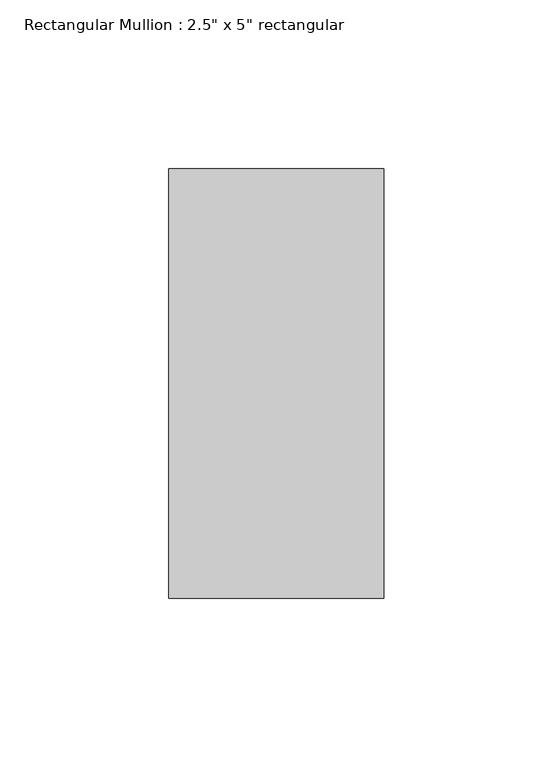
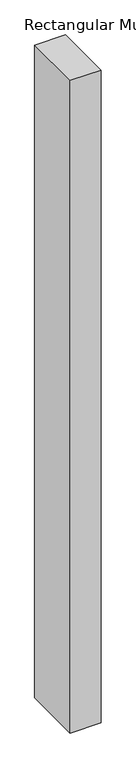
"""IFC4 building model written with IfcOpenShell, lengths in millimetres: member geometry."""

from ifc_helpers import new_model, si_unit, frame, origin, place, context, project, spatial, polyline, outline, extrude, source, transform, mapped, element, save


def member_3c30aa5e(model_context):
    return source(origin(), model_context, "Body", "SweptSolid", [
        extrude(outline(polyline([(31.75, 63.5), (31.75, -63.5), (-31.75, -63.5), (-31.75, 63.5), (31.75, 63.5)])), frame((0.0, 0.0, -1426.6333333), z_axis=(0.0, 0.0, 1.0), x_axis=(1.0, 0.0, 0.0)), (0.0, 0.0, 1.0), 1426.6333333),
    ])


if __name__ == "__main__":
    model = new_model("IFC4")
    model_context = context("Model", 3, world=origin())
    ifc_project = project(units=[si_unit("LENGTHUNIT", "METRE", prefix="MILLI")], contexts=[model_context])
    site = spatial("IfcSite", under=ifc_project)
    building = spatial("IfcBuilding", under=site)
    placement = place(None, origin())
    member_shape = member_3c30aa5e(model_context)
    element("IfcMember", 1, ObjectType="Rectangular Mullion : 2.5\" x 5\" rectangular", at=placement, inside=building, context=model_context, shape_type="MappedRepresentation", body=[
        mapped(member_shape, transform((0.0, 0.0, 0.0), x_axis=(1.0, 0.0, 0.0), y_axis=(0.0, 1.0, 0.0), z_axis=(0.0, 0.0, 1.0))),
    ])
    save(model, "model.ifc")

# Revit data of these elements
# Type "Rectangular Mullion : 2.5\" x 5\" rectangular"
#   built-in parameter 1007304 = 0.416667 (stored number, unit not read)
#   built-in parameter 1007301 = 0.104167 (stored number, unit not read)
#   built-in parameter 1007300 = 0.104167 (stored number, unit not read)
# Element 1 (IfcMember, "Rectangular Mullion : 2.5\" x 5\" rectangular")
#   Materials on its faces: "Aluminum"
# Materials
#   "Aluminum": class "Metal", colour RGB 247 247 247, transparency 0, Description = "Aluminum 6061", Cost = 0
